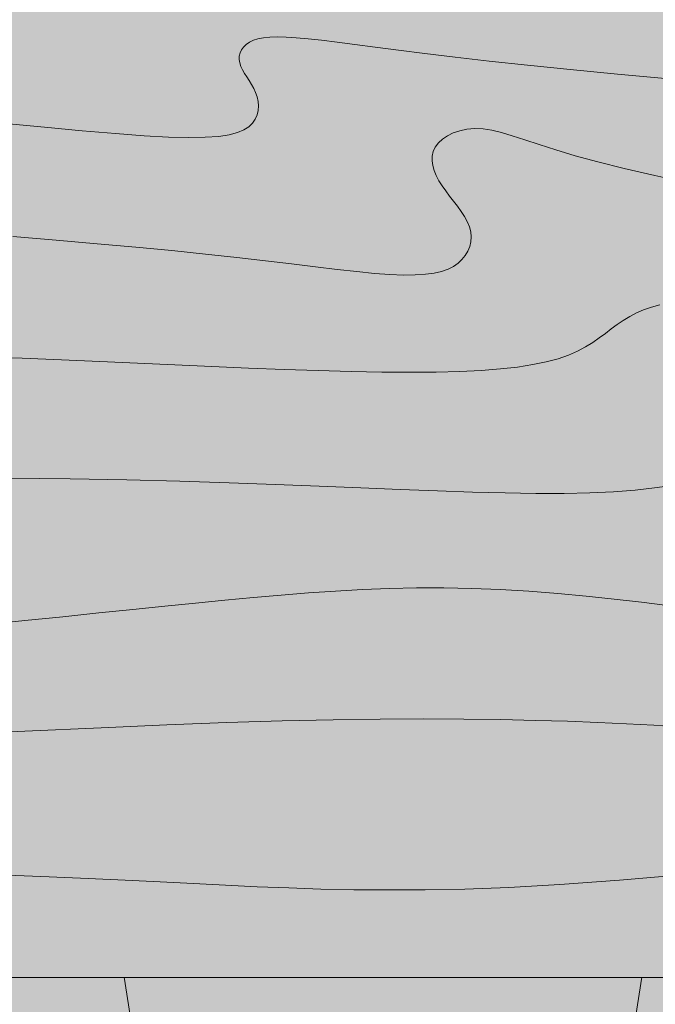
# Model space of a CAD drawing. Units: inches. Extents: x 3024 to 3952, y 1308 to 1863.
# Tile 10 of 29: x 3357 to 3374, y 1587 to 1613. Entities that reach past the tile are written whole.
import ezdxf

# ---------------------------------------------------------------- set-up
doc = ezdxf.new("R2010")
doc.units = ezdxf.units.IN
doc.layers.add('A-FLOR-PATT', color=254, linetype='Continuous', lineweight=13, true_color=0xfeeab9)
for name, color, linetype, lineweight in [('A-FLOR-TILE-PATT', 7, 'Continuous', 13), ('A-FURN', 8, 'Continuous', 18), ('A-FURN-PATT', 9, 'Continuous', 13)]:
    doc.layers.add(name, color=color, linetype=linetype, lineweight=lineweight)

# ---------------------------------------------------------------- blocks, each defined once
blk = doc.blocks.new('Dining Set - 36 x 72 in.')
for p, q in [((-36, -18), (36, -18)), ((5.7657, -26.0006), (4.5153, -17.99762)), ((23.4848, -17.99762), (22.2345, -25.99928))]:
    blk.add_line(p, q)
for points in [[(0.0365, 13.29166), (1.5945, 13.14388), (2.9811, 13.01562), (4.1988, 12.9108), (5.25, 12.83333), (6.1393, 12.78613), (6.8802, 12.76823), (7.4883, 12.77767), (7.9792, 12.8125), (8.3685, 12.87077), (8.6719, 12.95052), (8.9049, 13.0498), (9.0833, 13.16666), (9.2205, 13.29899), (9.3216, 13.44401), (9.3895, 13.59879), (9.4271, 13.76041), (9.4373, 13.92594), (9.4232, 14.09245), (9.3875, 14.257), (9.3333, 14.41666), (9.2638, 14.56917), (9.1836, 14.71484), (9.0975, 14.85465), (9.0104, 14.98958), (8.9272, 15.1206), (8.8529, 15.2487), (8.7922, 15.37483), (8.75, 15.5), (8.7305, 15.62467), (8.7344, 15.74739), (8.7617, 15.86621), (8.8125, 15.97916), (8.8867, 16.08431), (8.9844, 16.17968), (9.1055, 16.26334), (9.25, 16.33333), (9.4189, 16.38802), (9.6172, 16.42708), (9.8506, 16.45052), (10.125, 16.45833), (10.4463, 16.45052), (10.8203, 16.42708), (11.2529, 16.38802), (11.75, 16.33333), (12.3184, 16.26318), (12.9694, 16.17838), (13.7151, 16.07991), (14.5677, 15.96875), (15.5395, 15.84586), (16.6426, 15.71224), (17.8893, 15.56884), (19.2917, 15.41666), (20.859, 15.25667), (22.5879, 15.08984), (24.4721, 14.91715)], [(0.4415, 9.14534), (2.026, 9.01041), (3.5266, 8.87939), (4.9408, 8.7513), (6.266, 8.62516), (7.5, 8.5), (8.6411, 8.37549), (9.6914, 8.2539), (10.6538, 8.13818), (11.5312, 8.03125), (12.3267, 7.93603), (13.043, 7.85547), (13.6831, 7.79248), (14.25, 7.75), (14.7471, 7.7303), (15.1797, 7.73307), (15.5537, 7.75732), (15.875, 7.80208), (16.1494, 7.86637), (16.3828, 7.94922), (16.5811, 8.04964), (16.75, 8.16666), (16.8944, 8.29915), (17.0143, 8.44531), (17.1089, 8.60319), (17.1771, 8.77083), (17.218, 8.94629), (17.2305, 9.1276), (17.2137, 9.31282), (17.1667, 9.5), (17.0895, 9.6875), (16.987, 9.875), (16.8649, 10.0625), (16.7292, 10.25), (16.5856, 10.4375), (16.4401, 10.625), (16.2985, 10.8125), (16.1667, 11), (16.05, 11.18733), (15.9518, 11.3737), (15.8752, 11.5581), (15.8229, 11.73958), (15.798, 11.91715), (15.8034, 12.08984), (15.842, 12.25667), (15.9167, 12.41666), (16.0295, 12.56836), (16.1784, 12.70833), (16.3605, 12.83268), (16.5729, 12.9375), (16.8127, 13.01888), (17.0768, 13.07291), (17.3625, 13.0957), (17.6667, 13.08333), (17.9894, 13.03312), (18.3418, 12.94726), (18.7382, 12.82918), (19.1927, 12.68229), (19.7195, 12.51001), (20.3327, 12.31575), (21.0465, 12.10294), (21.875, 11.875), (22.8357, 11.63354), (23.959, 11.37304), (25.2786, 11.08618)], [(-0.7396, 4.73958), (0.7739, 4.6831), (2.22, 4.6237), (3.6213, 4.56233), (5, 4.5), (6.373, 4.43782), (7.7344, 4.3776), (9.0723, 4.32129), (10.375, 4.27083), (11.6309, 4.22819), (12.8281, 4.19531), (13.9551, 4.17415), (15, 4.16666), (15.954, 4.17448), (16.819, 4.19791), (17.6001, 4.23698), (18.3021, 4.29166), (18.9299, 4.36198), (19.4883, 4.44791), (19.9823, 4.54948), (20.4167, 4.66666), (20.7969, 4.79899), (21.1302, 4.94401), (21.4245, 5.09879), (21.6875, 5.26041), (21.9271, 5.42594), (22.1511, 5.59245), (22.3672, 5.757), (22.5834, 5.91666), (22.8065, 6.06868), (23.0404, 6.21093), (23.2879, 6.34147), (23.5521, 6.45833), (23.8358, 6.55957), (24.142, 6.64323)], [(0.2878, 0.28711), (2.5317, 0.26163), (4.6146, 0.22396), (6.5529, 0.17651), (8.3633, 0.12174), (10.0623, 0.06209), (11.6667, 0), (13.1899, -0.06201), (14.6341, -0.1211), (15.9982, -0.17432), (17.2813, -0.21875), (18.4823, -0.25147), (19.6003, -0.26953), (20.6343, -0.27002), (21.5834, -0.25), (22.4481, -0.20768), (23.2357, -0.14584), (23.9549, -0.06836), (24.6146, 0.02083)], [(-0.625, -5.08334), (0.8708, -4.93099), (2.2715, -4.78646), (3.5872, -4.64974), (4.8281, -4.52084), (6.0046, -4.39974), (7.127, -4.28646), (8.2053, -4.18099), (9.25, -4.08334), (10.2705, -3.99382), (11.2734, -3.91407), (12.2647, -3.84603), (13.25, -3.79167), (14.2354, -3.75293), (15.2266, -3.73177), (16.2295, -3.73015), (17.25, -3.75), (18.2912, -3.79248), (19.3451, -3.85547), (20.4009, -3.93604), (21.4479, -4.03125), (22.4754, -4.13819), (23.4727, -4.25391), (24.4289, -4.37549)], [(-2.5226, -9.12354), (0.8789, -8.98047), (3.6769, -8.85498), (6.0833, -8.75), (8.2767, -8.66765), (10.3021, -8.60677), (12.1712, -8.56543), (13.8958, -8.54167), (15.4876, -8.53353), (16.9583, -8.53907), (18.3197, -8.55632), (19.5834, -8.58334), (20.7616, -8.61841), (21.8685, -8.66081), (22.9188, -8.71004), (23.9271, -8.76563), (24.9081, -8.82707)], [(0.2448, -14.26042), (1.7647, -14.3169), (3.1973, -14.3763), (4.5507, -14.43767), (5.8333, -14.5), (7.0554, -14.5621), (8.235, -14.62175), (9.3922, -14.67652), (10.5469, -14.72396), (11.7192, -14.76164), (12.929, -14.78711), (14.1965, -14.79794), (15.5417, -14.79167), (16.9933, -14.76424), (18.6152, -14.70508), (20.4804, -14.60197), (22.6615, -14.44271), (25.2312, -14.21509), (28.2624, -13.9069), (31.8277, -13.50594), (36, -13)]]:
    blk.add_lwpolyline(points)

msp = doc.modelspace()

# ---------------------------------------------------------------- hatches: boundary and pattern name
at = {"layer": 'A-FLOR-PATT', "transparency": 33554528}
h = msp.add_hatch(color=256, dxfattribs=at)
h.dxf.hatch_style = 1
h.paths.add_polyline_path([(3460.764, 1688.6064), (3412.764, 1688.6064), (3412.764, 1694.6064), (3460.764, 1694.6064), (3460.764, 1778.6064), (3406.764, 1778.6064), (3406.764, 1759.9514), (3318.2981, 1759.9514), (3318.2981, 1658.6064), (3322.5356, 1658.6064), (3322.5356, 1652.6064), (3292.764, 1652.6064), (3292.764, 1778.6064), (3106.764, 1778.6064), (3106.764, 1628.6064), (3172.764, 1628.6064), (3172.764, 1532.6064), (3166.764, 1532.6064), (3166.764, 1628.6064), (3106.764, 1628.6064), (3106.764, 1356.8452), (3202.812, 1356.8452), (3202.812, 1354.2534), (3202.812, 1353.8388), (3202.812, 1351.1212), (3202.812, 1347.8452), (3277.764, 1347.8452), (3277.764, 1353.8452), (3277.764, 1356.8452), (3277.764, 1442.6064), (3460.764, 1442.6064)])
h.paths.add_polyline_path([(3216.238, 1527.2064), (3216.238, 1491.2064), (3214.663, 1491.2064), (3214.663, 1491.2409, -0.3966224), (3180.243, 1526.6064), (3163.0285, 1526.6064), (3163.0285, 1531.1064), (3161.716, 1531.1064), (3161.716, 1561.1064), (3163.0285, 1561.1064), (3163.0285, 1531.1064), (3163.0285, 1526.6064), (3180.243, 1526.6064, 0.3966224), (3214.663, 1491.2409), (3214.663, 1527.2064)], flags=16)
h.paths.add_polyline_path([(3227.364, 1649.8972), (3191.364, 1649.8972), (3191.364, 1651.4722), (3227.364, 1651.4722)], flags=16)
h.paths.add_polyline_path([(3323.1172, 1606.7362), (3323.8545, 1606.8514), (3323.8545, 1594.8241), (3323.1172, 1594.9393)], flags=16)
h.paths.add_polyline_path([(3324.2232, 1606.909), (3330.1216, 1607.8307), (3330.1216, 1614.1093), (3339.3495, 1614.1093), (3340.2711, 1620.0078), (3352.4136, 1620.0078), (3353.3353, 1614.1093), (3359.9941, 1614.1093), (3360.9157, 1620.0078), (3373.0582, 1620.0078), (3373.9799, 1614.1093), (3383.2077, 1614.1093), (3383.2077, 1607.8307), (3389.1062, 1606.909), (3389.1062, 1594.7665), (3383.2077, 1593.8449), (3383.2077, 1587.5663), (3373.9799, 1587.5663), (3373.0583, 1581.6678), (3360.9157, 1581.6678), (3359.9941, 1587.5663), (3353.3353, 1587.5663), (3352.4136, 1581.6678), (3340.2711, 1581.6678), (3339.3495, 1587.5663), (3330.1216, 1587.5663), (3330.1216, 1593.8449), (3324.2232, 1594.7665)], flags=16)
h.paths.add_polyline_path([(3236.1584, 1693.1064), (3236.1584, 1723.1064), (3237.4709, 1723.1064), (3237.4709, 1693.1064)], flags=16)
h.paths.add_polyline_path([(3373.2158, 1600.6847), (3373.7965, 1600.7303), (3374.3268, 1600.7874), (3374.8132, 1600.8531), (3375.2621, 1600.9247), (3375.6801, 1600.9991), (3376.0736, 1601.0735), (3376.6855, 1601.19), (3377.366, 1601.3023), (3378.0667, 1601.3814), (3378.8026, 1601.4123), (3379.5865, 1601.3839), (3380.4537, 1601.2948), (3381.301, 1601.1717), (3382.0317, 1601.0433), (3382.4398, 1600.9607), (3382.6252, 1600.9201), (3382.919, 1600.8507), (3382.9044, 1600.8531), (3382.842, 1600.8678), (3382.7541, 1600.8896), (3382.6252, 1600.9201), (3382.4398, 1600.9607), (3382.1868, 1601.0119), (3381.8738, 1601.0711), (3381.5125, 1601.1346), (3381.1149, 1601.1988), (3380.6928, 1601.2601), (3380.2581, 1601.3149), (3379.8226, 1601.3597), (3379.3984, 1601.3908), (3378.9944, 1601.4054), (3378.6092, 1601.4042), (3378.2384, 1601.3886), (3377.8777, 1601.36), (3377.5227, 1601.32), (3377.1691, 1601.2698), (3376.8127, 1601.211), (3376.4491, 1601.145), (3376.0736, 1601.0735), (3375.4177, 1600.9494), (3374.5542, 1600.8119), (3373.5044, 1600.6988)], flags=0)
h.paths.add_polyline_path([(3380.0253, 1596.7351), (3380.499, 1596.6659), (3380.9706, 1596.6119), (3381.4375, 1596.5791), (3381.8971, 1596.5736), (3382.5886, 1596.6167), (3382.7848, 1596.6692), (3382.1465, 1596.5706), (3381.236, 1596.5815), (3380.3199, 1596.6865)], flags=0)
h.paths.add_polyline_path([(3369.6414, 1603.9617), (3370.1589, 1604.0021), (3370.6218, 1604.0539), (3371.0335, 1604.1173), (3371.3978, 1604.1921), (3371.7181, 1604.2785), (3371.9984, 1604.3761), (3372.2441, 1604.483), (3372.4611, 1604.5972), (3372.655, 1604.7163), (3372.8317, 1604.8384), (3372.9968, 1604.9611), (3373.3703, 1605.2455), (3373.8426, 1605.5328), (3374.4624, 1605.7539), (3375.1058, 1605.8302), (3375.7221, 1605.8261), (3376.4109, 1605.76), (3377.1534, 1605.6376), (3377.8945, 1605.473), (3378.1382, 1605.409), (3377.7394, 1605.5074), (3377.3509, 1605.5937), (3376.9704, 1605.6677), (3376.5999, 1605.7288), (3376.2417, 1605.7762), (3375.8979, 1605.8092), (3375.5707, 1605.8271), (3375.2621, 1605.8291), (3374.9745, 1605.8146), (3374.7092, 1605.7832), (3374.4647, 1605.7359), (3374.239, 1605.6742), (3374.0298, 1605.5996), (3373.835, 1605.5134), (3373.6525, 1605.4171), (3373.4801, 1605.3123), (3373.3156, 1605.2002), (3373.1562, 1605.0825), (3372.7603, 1604.781), (3372.236, 1604.4588), (3371.5738, 1604.2283), (3370.8493, 1604.0794), (3369.9262, 1603.976)], flags=0)
h.paths.add_polyline_path([(3366.7533, 1606.5832), (3367.1713, 1606.5519), (3367.5378, 1606.5374), (3367.8568, 1606.5394), (3368.1325, 1606.5573), (3368.3694, 1606.5903), (3368.5717, 1606.6377), (3368.7438, 1606.6988), (3368.89, 1606.7728), (3369.0146, 1606.8591), (3369.121, 1606.9568), (3369.2094, 1607.0646), (3369.2792, 1607.181), (3369.3295, 1607.3046), (3369.3596, 1607.4339), (3369.3688, 1607.5676), (3369.3565, 1607.7042), (3369.3218, 1607.8422), (3369.2649, 1607.9804), (3369.1893, 1608.1187), (3369.0993, 1608.2569), (3368.9992, 1608.3952), (3368.8934, 1608.5334), (3368.7861, 1608.6717), (3368.6817, 1608.8099), (3368.4212, 1609.1804), (3368.2685, 1609.7106), (3368.4883, 1610.1814), (3369.0537, 1610.4604), (3369.6717, 1610.5097), (3370.2812, 1610.3612), (3370.4805, 1610.2968), (3370.1882, 1610.3839), (3369.9284, 1610.4472), (3369.6905, 1610.4842), (3369.4662, 1610.4933), (3369.2555, 1610.4765), (3369.0608, 1610.4367), (3368.884, 1610.3767), (3368.7274, 1610.2994), (3368.5931, 1610.2077), (3368.4833, 1610.1045), (3368.4002, 1609.9927), (3368.3451, 1609.8747), (3368.3166, 1609.7517), (3368.3127, 1609.6244), (3368.331, 1609.4935), (3368.3696, 1609.3597), (3368.4261, 1609.2237), (3368.4985, 1609.0863), (3368.5845, 1608.9482), (3368.6817, 1608.8099), (3368.7861, 1608.6717), (3368.8934, 1608.5334), (3368.9992, 1608.3952), (3369.0993, 1608.2569), (3369.3398, 1607.8876), (3369.3941, 1607.2896), (3368.9774, 1606.7817), (3368.3928, 1606.5742), (3367.7162, 1606.5303), (3367.0044, 1606.5585)], flags=0)
h.paths.add_polyline_path([(3362.1859, 1610.2589), (3362.5478, 1610.2845), (3362.8348, 1610.3275), (3363.0585, 1610.3863), (3363.2303, 1610.4595), (3363.3619, 1610.5457), (3363.463, 1610.6432), (3363.5376, 1610.7502), (3363.5876, 1610.8643), (3363.6153, 1610.9834), (3363.6229, 1611.1055), (3363.6125, 1611.2283), (3363.5861, 1611.3496), (3363.5462, 1611.4673), (3363.4949, 1611.5797), (3363.4358, 1611.6871), (3363.3723, 1611.7902), (3363.3081, 1611.8897), (3363.2468, 1611.9863), (3363.192, 1612.0808), (3363.0258, 1612.4261), (3363.3371, 1612.8672), (3363.9008, 1612.9782), (3364.4822, 1612.9641), (3365.1098, 1612.9074), (3365.328, 1612.8805), (3364.9615, 1612.9208), (3364.6426, 1612.9496), (3364.3668, 1612.9669), (3364.1299, 1612.9726), (3363.9276, 1612.9669), (3363.7555, 1612.9496), (3363.6093, 1612.9208), (3363.4848, 1612.8805), (3363.3782, 1612.8289), (3363.2889, 1612.7672), (3363.2169, 1612.6969), (3363.1622, 1612.6193), (3363.1247, 1612.5361), (3363.1046, 1612.4484), (3363.1017, 1612.358), (3363.1161, 1612.266), (3363.1472, 1612.1738), (3363.192, 1612.0808), (3363.2468, 1611.9863), (3363.3081, 1611.8897), (3363.3723, 1611.7902), (3363.4358, 1611.6871), (3363.6363, 1611.323), (3363.5979, 1610.7003), (3363.0863, 1610.3651), (3362.3983, 1610.2622)], flags=0)
h.paths.add_polyline_path([(3352.356, 1581.2991), (3352.2408, 1580.5618), (3340.4439, 1580.5618), (3340.3287, 1581.2991)], flags=16)
h.paths.add_polyline_path([(3340.4439, 1621.1137), (3352.2408, 1621.1137), (3352.356, 1620.3764), (3340.3287, 1620.3764)], flags=16)
h.paths.add_polyline_path([(3278.4282, 1504.7424), (3290.3831, 1504.7424), (3290.3831, 1502.7499), (3291.0473, 1502.7499), (3291.0473, 1494.7799), (3290.3831, 1494.7799), (3290.3831, 1494.1158), (3291.0473, 1494.1158), (3291.0473, 1486.1458), (3290.3831, 1486.1458), (3290.3831, 1484.1533), (3291.0473, 1484.1533), (3291.0473, 1483.4892, -0.0909091), (3291.0473, 1468.8776), (3291.0473, 1468.2135), (3290.3831, 1468.2135), (3290.3831, 1464.8926), (3278.4282, 1464.8926), (3278.4282, 1472.8626), (3277.764, 1473.5268), (3277.764, 1478.84), (3278.4282, 1479.5042)], flags=16)
h.paths.add_polyline_path([(3278.7603, 1504.4103), (3290.051, 1504.4103), (3290.051, 1465.2247), (3278.7603, 1465.2247)], flags=0)
h.paths.add_polyline_path([(3123.904, 1600.7821), (3117.9039, 1602.7821), (3117.9039, 1599.7821), (3119.4039, 1599.7821), (3119.4039, 1596.7821), (3118.4039, 1596.7821), (3118.4039, 1598.7821), (3117.9039, 1598.7821), (3117.9039, 1596.2821), (3109.9039, 1596.2821), (3109.9039, 1617.2821), (3117.9039, 1617.2821), (3117.9039, 1610.7821), (3123.9038, 1612.7821, -0.7025712), (3137.9039, 1606.7822, -0.7025621)], flags=16)
h.paths.add_polyline_path([(3123.9039, 1602.7822), (3123.9039, 1610.7822, -0.7345333), (3136.9039, 1606.7822, -0.7345297)], flags=0)
h.paths.add_polyline_path([(3177.972, 1689.6473), (3109.2405, 1689.6473), (3109.2405, 1741.1959), (3177.972, 1741.1959)], flags=16)
h.paths.add_polyline_path([(3373.0006, 1581.2991), (3372.8854, 1580.5618), (3361.0885, 1580.5618), (3360.9733, 1581.2991)], flags=16)
h.paths.add_polyline_path([(3361.0885, 1621.1137), (3372.8854, 1621.1137), (3373.0006, 1620.3764), (3360.9733, 1620.3764)], flags=16)
h.paths.add_polyline_path([(3116.9039, 1598.2821, -0.4142136), (3116.1539, 1597.2821), (3111.9039, 1597.2821, -0.4142136), (3110.9039, 1598.0321), (3110.9039, 1615.2821, -0.4142136), (3111.6539, 1616.2821), (3115.9039, 1616.2821, -0.4142136), (3116.9039, 1615.5321)], flags=0)
h.paths.add_polyline_path([(3121.6122, 1728.1369), (3121.6122, 1696.5205), (3110.2715, 1696.5205), (3110.2715, 1714.3906), (3121.6122, 1714.3906), (3121.6122, 1716.4526), (3110.2715, 1716.4526), (3110.2715, 1734.3228), (3123.3304, 1734.3228), (3123.3304, 1729.8552), (3134.6711, 1741.1959), (3134.6711, 1728.1369)], flags=0)
h.paths.add_polyline_path([(3389.4748, 1606.8514), (3390.2122, 1606.7362), (3390.2122, 1594.9393), (3389.4748, 1594.8241)], flags=16)
h.paths.add_polyline_path([(3257.6842, 1762.8281), (3259.6842, 1768.8281), (3256.6842, 1768.8281), (3256.6842, 1767.3281), (3253.6842, 1767.3281), (3253.6842, 1768.3281), (3255.6842, 1768.3281), (3255.6842, 1768.8281), (3253.1842, 1768.8281), (3253.1842, 1776.8281), (3274.1842, 1776.8281), (3274.1842, 1768.8281), (3267.6842, 1768.8281), (3269.6842, 1762.8282, -0.7025712), (3263.6843, 1748.8282, -0.7025621)], flags=16)
h.paths.add_polyline_path([(3259.6842, 1762.8281), (3267.6843, 1762.8281, -0.7345333), (3263.6842, 1749.8282, -0.7345297)], flags=0)
h.paths.add_polyline_path([(3411.264, 1715.6064), (3411.264, 1716.9189), (3441.264, 1716.9189), (3441.264, 1715.6064)], flags=16)
h.paths.add_polyline_path([(3178.3806, 1449.1876), (3178.3806, 1397.639), (3109.6491, 1397.639), (3109.6491, 1449.1876)], flags=16)
h.paths.add_polyline_path([(3397.1501, 1541.7146), (3419.6183, 1541.7146), (3419.6183, 1496.7783), (3397.1501, 1496.7783)], flags=16)
h.paths.add_polyline_path([(3254.1842, 1770.5781), (3254.1842, 1774.8281, -0.4142136), (3254.9342, 1775.8281), (3272.1842, 1775.8281, -0.4142136), (3273.1842, 1775.0781), (3273.1842, 1770.8281, -0.4142136), (3272.4342, 1769.8281), (3255.1842, 1769.8281, -0.4142136)], flags=0)
h.paths.add_polyline_path([(3403.672, 1500.7601), (3403.6016, 1500.3997), (3403.5328, 1500.0441), (3403.4662, 1499.6867), (3403.4027, 1499.3226), (3403.3464, 1498.9532), (3403.3025, 1498.5811), (3403.2759, 1498.2091), (3403.2714, 1497.8401), (3403.3064, 1497.2813), (3403.3491, 1497.1219), (3403.2689, 1497.6395), (3403.2778, 1498.3719), (3403.3635, 1499.0984), (3403.4889, 1499.8168), (3403.6016, 1500.3997), (3403.672, 1500.7601), (3403.744, 1501.1315), (3403.817, 1501.5205), (3403.891, 1501.9336), (3403.9656, 1502.3769), (3404.0404, 1502.8572), (3404.115, 1503.3786), (3404.2264, 1504.2311), (3404.2571, 1504.5223), (3404.1552, 1503.6598), (3404.0063, 1502.6193), (3403.8604, 1501.7518), (3403.744, 1501.1315)], flags=0)
h.paths.add_polyline_path([(3406.5868, 1505.0416), (3406.6121, 1504.5236), (3406.6492, 1504.0526), (3406.6956, 1503.624), (3406.7491, 1503.2333), (3406.8072, 1502.8759), (3406.8676, 1502.5473), (3406.9281, 1502.243), (3407.0268, 1501.7597), (3407.1416, 1501.1368), (3407.2087, 1500.3904), (3407.1804, 1499.6703), (3407.1078, 1498.9956), (3407.0074, 1498.3199), (3406.8809, 1497.6059), (3406.7403, 1496.9627), (3406.7418, 1496.9824), (3406.7491, 1497.0249), (3406.8229, 1497.3409), (3406.8364, 1497.4025), (3406.878, 1497.6078), (3406.9261, 1497.8614), (3406.9777, 1498.1526), (3407.0298, 1498.4712), (3407.0797, 1498.8068), (3407.1243, 1499.149), (3407.1607, 1499.4874), (3407.1859, 1499.8115), (3407.1978, 1500.1137), (3407.1969, 1500.3962), (3407.1841, 1500.6642), (3407.1609, 1500.9225), (3407.1284, 1501.1761), (3407.0876, 1501.43), (3407.0398, 1501.6891), (3406.9862, 1501.9585), (3406.8832, 1502.4628), (3406.7712, 1503.0713), (3406.6657, 1503.8424), (3406.5924, 1504.7735)], flags=0)
h.paths.add_polyline_path([(3409.2517, 1507.8962), (3409.2752, 1507.4282), (3409.3079, 1507.0076), (3409.3501, 1506.6314), (3409.4015, 1506.2969), (3409.4624, 1506.0009), (3409.5326, 1505.7406), (3409.6119, 1505.5128), (3409.6988, 1505.3131), (3409.7915, 1505.1368), (3409.8883, 1504.9792), (3409.9875, 1504.8356), (3410.0872, 1504.7015), (3410.1859, 1504.572), (3410.4508, 1504.2132), (3410.7205, 1503.6035), (3410.8059, 1502.8824), (3410.7619, 1502.0875), (3410.6122, 1501.2299), (3410.4402, 1500.6169), (3410.2538, 1500.0031), (3410.0536, 1499.3219), (3409.9909, 1499.0812), (3410.1761, 1499.7472), (3410.3596, 1500.3513), (3410.4512, 1500.6561), (3410.5312, 1500.9412), (3410.6013, 1501.226), (3410.6614, 1501.512), (3410.7111, 1501.7964), (3410.7496, 1502.0763), (3410.7764, 1502.3489), (3410.7909, 1502.6114), (3410.7926, 1502.8608), (3410.7808, 1503.0944), (3410.7553, 1503.31), (3410.7169, 1503.5087), (3410.6667, 1503.6921), (3410.6061, 1503.8621), (3410.5361, 1504.0203), (3410.4578, 1504.1686), (3410.3726, 1504.3088), (3410.2815, 1504.4424), (3410.1859, 1504.572), (3410.0872, 1504.7015), (3409.859, 1505.0083), (3409.5943, 1505.5117), (3409.4266, 1506.1336), (3409.324, 1506.8011), (3409.2586, 1507.6407)], flags=0)
h.paths.add_polyline_path([(3411.4914, 1510.5878), (3411.4432, 1510.1586), (3411.4054, 1509.775), (3411.38, 1509.4354), (3411.3681, 1509.1376), (3411.3698, 1508.8784), (3411.3843, 1508.6542), (3411.4112, 1508.4618), (3411.4497, 1508.2974), (3411.4994, 1508.1575), (3411.5595, 1508.0388), (3411.6296, 1507.9375), (3411.7097, 1507.851), (3411.802, 1507.7792), (3411.9096, 1507.7225), (3412.0353, 1507.6817), (3412.1821, 1507.6572), (3412.3528, 1507.6496), (3412.5505, 1507.6597), (3412.778, 1507.6879), (3413.0364, 1507.7341), (3413.3194, 1507.7955), (3413.6188, 1507.8687), (3413.9264, 1507.95), (3414.234, 1508.036), (3414.5333, 1508.1232), (3414.8163, 1508.208), (3415.0747, 1508.287), (3415.3023, 1508.3569), (3415.5007, 1508.4158), (3415.6733, 1508.4617), (3416.1158, 1508.5538), (3416.512, 1508.2591), (3416.716, 1507.6581), (3416.61, 1507.0003), (3416.3052, 1506.3411), (3415.8928, 1505.618), (3415.7339, 1505.3633), (3415.9914, 1505.791), (3416.201, 1506.1583), (3416.3666, 1506.4739), (3416.4925, 1506.7462), (3416.5828, 1506.9838), (3416.6413, 1507.1949), (3416.6725, 1507.3883), (3416.6799, 1507.5705), (3416.6662, 1507.7417), (3416.6339, 1507.9), (3416.5851, 1508.0436), (3416.5223, 1508.1709), (3416.4478, 1508.28), (3416.3639, 1508.3692), (3416.273, 1508.4368), (3416.1765, 1508.4815), (3416.0718, 1508.5047), (3415.9553, 1508.5079), (3415.8237, 1508.493), (3415.6733, 1508.4617), (3415.5007, 1508.4158), (3415.3327, 1508.3659), (3414.6495, 1508.157), (3414.0606, 1507.9855), (3413.4456, 1507.8229), (3412.8838, 1507.701), (3412.5505, 1507.6597), (3412.0748, 1507.6354), (3411.595, 1507.8883), (3411.398, 1508.4429), (3411.3624, 1508.9927), (3411.3854, 1509.5711), (3411.4578, 1510.3071)], flags=0)
h.paths.add_polyline_path([(3135.0797, 1449.1876), (3135.0797, 1436.1286), (3122.0208, 1436.1286), (3122.0208, 1404.5122), (3110.6801, 1404.5122), (3110.6801, 1422.3823), (3122.0208, 1422.3823), (3122.0208, 1424.4443), (3110.6801, 1424.4443), (3110.6801, 1442.3145), (3123.739, 1442.3145), (3123.739, 1437.8469)], flags=0)
h.paths.add_polyline_path([(3416.4944, 1514.2949), (3416.4837, 1513.8511), (3416.4893, 1513.4867), (3416.5102, 1513.1926), (3416.5451, 1512.9593), (3416.5929, 1512.7775), (3416.6524, 1512.6379), (3416.7224, 1512.531), (3416.8017, 1512.4488), (3416.8886, 1512.3882), (3416.9813, 1512.3476), (3417.0781, 1512.3251), (3417.1773, 1512.3189), (3417.277, 1512.3274), (3417.3757, 1512.3488), (3417.4713, 1512.3813), (3417.5627, 1512.4229), (3417.65, 1512.471), (3417.7338, 1512.5225), (3417.8146, 1512.5747), (3417.8931, 1512.6245), (3417.9699, 1512.6691), (3418.2968, 1512.8265), (3418.6505, 1512.4645), (3418.7037, 1511.9342), (3418.6693, 1511.3839), (3418.6076, 1510.8228), (3418.5777, 1510.5927), (3418.6197, 1510.9333), (3418.6525, 1511.2311), (3418.6759, 1511.4903), (3418.6899, 1511.7144), (3418.6946, 1511.9069), (3418.6899, 1512.0713), (3418.6759, 1512.2112), (3418.6525, 1512.33), (3418.6197, 1512.4311), (3418.5778, 1512.5177), (3418.5276, 1512.5903), (3418.4705, 1512.6488), (3418.4075, 1512.6933), (3418.3399, 1512.7237), (3418.2686, 1512.7401), (3418.1951, 1512.7424), (3418.1204, 1512.7307), (3418.0455, 1512.7055), (3417.9792, 1512.6736), (3417.65, 1512.471), (3417.5627, 1512.4229), (3417.4713, 1512.3813), (3417.3757, 1512.3488), (3417.277, 1512.3274), (3416.878, 1512.2936), (3416.5757, 1512.7549), (3416.492, 1513.3145), (3416.4808, 1514.0384)], flags=0)
h.paths.add_polyline_path([(3392.8223, 1481.9454), (3396.7707, 1481.9454), (3396.7707, 1480.9201), (3428.3585, 1480.9201), (3428.3585, 1481.9454), (3432.3069, 1481.9454), (3432.3069, 1464.8354, -0.266667), (3392.8223, 1464.8354)], flags=16)
h.paths.add_polyline_path([(3431.203, 1547.5428), (3450.8613, 1547.5428, -0.1904762), (3450.8614, 1484.031), (3431.203, 1484.031), (3431.203, 1488.5675), (3432.3809, 1488.5675), (3432.3809, 1543.0062), (3431.203, 1543.0062)], flags=16)
h.paths.add_polyline_path([(3451.9233, 1524.86, -0.0496282), (3451.9233, 1506.7138), (3446.7921, 1506.7138), (3446.7921, 1524.86)], flags=0)
h.paths.add_polyline_path([(3460.764, 1436.6064), (3277.764, 1436.6064), (3277.764, 1356.8452), (3277.764, 1353.8452), (3460.764, 1353.8452)], flags=17)
h.paths.add_polyline_path([(3121.3033, 1577.378), (3153.693, 1577.378), (3153.693, 1586.6752), (3121.3033, 1586.6752)], flags=24)
h.paths.add_polyline_path([(3164.1457, 1464.1276), (3210.4801, 1464.1276), (3210.4801, 1473.4247), (3164.1457, 1473.4247)], flags=24)
h.paths.add_polyline_path([(3343.1909, 1505.8863), (3373.7236, 1505.8863), (3373.7236, 1515.1773), (3343.1909, 1515.1773)], flags=24)
h.paths.add_polyline_path([(3337.6353, 1564.2926), (3370.0189, 1564.2926), (3370.0189, 1573.5836), (3337.6353, 1573.5836)], flags=24)
h.paths.add_polyline_path([(3419.204, 1753.8578), (3453.3997, 1753.8578), (3453.3997, 1762.9956), (3419.204, 1762.9956)], flags=24)
h.paths.add_polyline_path([(3341.2523, 1701.0246), (3381.0761, 1701.0246), (3381.0761, 1710.3156), (3341.2523, 1710.3156)], flags=24)
h.paths.add_polyline_path([(3245.8895, 1726.2997), (3278.2793, 1726.2997), (3278.2793, 1735.5968), (3245.8895, 1735.5968)], flags=24)
h.paths.add_polyline_path([(3128.8045, 1668.6736), (3175.1389, 1668.6736), (3175.1389, 1677.9707), (3128.8045, 1677.9707)], flags=24)
h.paths.add_polyline_path([(3345.9997, 1396.0062), (3389.09, 1396.0062), (3389.09, 1405.3033), (3345.9997, 1405.3033)], flags=24)
at = {"layer": 'A-FLOR-TILE-PATT', "transparency": 33554569}
h = msp.add_hatch(dxfattribs=at)
h.set_pattern_fill('ANGLE', color=256, scale=2)
h.set_pattern_definition([(0, (0, 0), (0, 13.97), [10.16, -3.81]), (90, (0, 0), (-13.97, 9e-16), [10.16, -3.81])])
h.paths.add_polyline_path([(3292.764, 1778.6064), (3232.764, 1778.6064), (3232.764, 1694.6064), (3236.1584, 1694.6064), (3236.1584, 1723.1064), (3237.4709, 1723.1064), (3237.4709, 1723.0777, -0.3870039), (3266.1209, 1694.6064), (3292.764, 1694.6064)])
h.paths.add_polyline_path([(3263.6843, 1748.8282, -0.7025621), (3257.6842, 1762.8281), (3259.6842, 1768.8281), (3256.6842, 1768.8281), (3256.6842, 1767.3281), (3253.6842, 1767.3281), (3253.6842, 1768.3281), (3255.6842, 1768.3281), (3255.6842, 1768.8281), (3253.1842, 1768.8281), (3253.1842, 1776.8281), (3274.1842, 1776.8281), (3274.1842, 1768.8281), (3267.6842, 1768.8281), (3269.6842, 1762.8282, -0.7025712)], flags=16)
h.paths.add_polyline_path([(3263.6842, 1749.8282, -0.7345297), (3259.6842, 1762.8281), (3267.6843, 1762.8281, -0.7345333)], flags=0)
h.paths.add_polyline_path([(3255.1842, 1769.8281, -0.4142136), (3254.1842, 1770.5781), (3254.1842, 1774.8281, -0.4142136), (3254.9342, 1775.8281), (3272.1842, 1775.8281, -0.4142136), (3273.1842, 1775.0781), (3273.1842, 1770.8281, -0.4142136), (3272.4342, 1769.8281)], flags=0)
h.paths.add_polyline_path([(3460.764, 1436.6064), (3277.764, 1436.6064), (3277.764, 1356.8452), (3277.764, 1353.8452), (3460.764, 1353.8452)])
h.paths.add_polyline_path([(3166.764, 1628.6064), (3106.764, 1628.6064), (3106.764, 1532.6064), (3133.066, 1532.6064, -0.3870039), (3161.716, 1561.0777), (3161.716, 1561.1064), (3163.0285, 1561.1064), (3163.0285, 1532.6064), (3166.764, 1532.6064)])
h.paths.add_polyline_path([(3123.904, 1600.7821), (3117.9039, 1602.7821), (3117.9039, 1599.7821), (3119.4039, 1599.7821), (3119.4039, 1596.7821), (3118.4039, 1596.7821), (3118.4039, 1598.7821), (3117.9039, 1598.7821), (3117.9039, 1596.2821), (3109.9039, 1596.2821), (3109.9039, 1617.2821), (3117.9039, 1617.2821), (3117.9039, 1610.7821), (3123.9038, 1612.7821, -0.7025712), (3137.9039, 1606.7822, -0.7025621)], flags=16)
h.paths.add_polyline_path([(3123.9039, 1602.7822), (3123.9039, 1610.7822, -0.7345333), (3136.9039, 1606.7822, -0.7345297)], flags=0)
h.paths.add_polyline_path([(3116.1539, 1597.2821), (3111.9039, 1597.2821, -0.4142136), (3110.9039, 1598.0321), (3110.9039, 1615.2821, -0.4142136), (3111.6539, 1616.2821), (3115.9039, 1616.2821, -0.4142136), (3116.9039, 1615.5321), (3116.9039, 1598.2821, -0.4142136)], flags=0)
h.paths.add_polyline_path([(3245.8895, 1726.2997), (3278.2793, 1726.2997), (3278.2793, 1735.5968), (3245.8895, 1735.5968)], flags=24)
h.paths.add_polyline_path([(3345.9997, 1396.0062), (3389.09, 1396.0062), (3389.09, 1405.3033), (3345.9997, 1405.3033)], flags=24)
h.paths.add_polyline_path([(3121.3033, 1577.378), (3153.693, 1577.378), (3153.693, 1586.6752), (3121.3033, 1586.6752)], flags=24)
at = {"layer": 'A-FURN-PATT', "transparency": 33554511}
h = msp.add_hatch(color=256, dxfattribs=at)
h.dxf.hatch_style = 1
h.paths.add_polyline_path([(3373.0582, 1620.0078), (3360.9157, 1620.0078), (3359.9941, 1614.1093), (3373.9799, 1614.1093)])
h.paths.add_polyline_path([(3372.8854, 1621.1137), (3361.0885, 1621.1137), (3360.9733, 1620.3764), (3373.0006, 1620.3764)])
h.paths.add_polyline_path([(3389.1062, 1606.909), (3383.2077, 1607.8307), (3383.2077, 1593.8449), (3389.1062, 1594.7665)])
h.paths.add_polyline_path([(3390.2122, 1606.7362), (3389.4748, 1606.8514), (3389.4748, 1594.8241), (3390.2122, 1594.9393)])
h.paths.add_polyline_path([(3373.9799, 1587.5663), (3359.9941, 1587.5663), (3360.9157, 1581.6678), (3373.0583, 1581.6678)])
h.paths.add_polyline_path([(3373.0006, 1581.2991), (3360.9733, 1581.2991), (3361.0885, 1580.5618), (3372.8854, 1580.5618)])
h.paths.add_polyline_path([(3353.3353, 1587.5663), (3339.3495, 1587.5663), (3340.2711, 1581.6678), (3352.4136, 1581.6678)])
h.paths.add_polyline_path([(3352.356, 1581.2991), (3340.3287, 1581.2991), (3340.4439, 1580.5618), (3352.2408, 1580.5618)])
h.paths.add_polyline_path([(3330.1216, 1607.8307), (3324.2232, 1606.909), (3324.2232, 1594.7665), (3330.1216, 1593.8449)])
h.paths.add_polyline_path([(3323.8545, 1606.8514), (3323.1172, 1606.7362), (3323.1172, 1594.9393), (3323.8545, 1594.8241)])
h.paths.add_polyline_path([(3352.4136, 1620.0078), (3340.2711, 1620.0078), (3339.3495, 1614.1093), (3353.3353, 1614.1093)])
h.paths.add_polyline_path([(3352.2408, 1621.1137), (3340.4439, 1621.1137), (3340.3287, 1620.3764), (3352.356, 1620.3764)])
at = {"layer": 'A-FURN-PATT', "transparency": 33554600}
h = msp.add_hatch(color=256, dxfattribs=at)
h.dxf.hatch_style = 1
h.paths.add_polyline_path([(3363.5462, 1611.4673), (3363.4949, 1611.5797), (3363.4358, 1611.6871), (3363.3723, 1611.7902), (3363.2557, 1611.9708), (3363.16, 1612.1359), (3363.1003, 1612.3129), (3363.1061, 1612.4946), (3363.1815, 1612.6623), (3363.3264, 1612.8038), (3363.5397, 1612.9071), (3363.7555, 1612.9496), (3363.9276, 1612.9669), (3364.1299, 1612.9726), (3364.3668, 1612.9669), (3364.6426, 1612.9496), (3364.9615, 1612.9208), (3365.328, 1612.8805), (3365.7471, 1612.8287), (3366.2271, 1612.7662), (3366.7769, 1612.6936), (3367.4055, 1612.6117), (3368.1221, 1612.5211), (3368.9354, 1612.4225), (3369.8546, 1612.3168), (3370.8886, 1612.2046), (3372.0442, 1612.0866), (3373.3189, 1611.9636), (3374.7081, 1611.8363), (3376.2072, 1611.7054), (3377.8113, 1611.5716), (3379.516, 1611.4356), (3381.3163, 1611.2982), (3383.2077, 1611.1601), (3383.2077, 1614.1093), (3330.1216, 1614.1093), (3330.1216, 1611.8974), (3333.6775, 1611.8808), (3336.899, 1611.834), (3339.8144, 1611.7613), (3342.4523, 1611.667), (3344.8411, 1611.5554), (3347.0091, 1611.4308), (3348.985, 1611.2976), (3350.797, 1611.1601), (3352.4691, 1611.0223), (3354.0078, 1610.8874), (3355.4146, 1610.7583), (3356.6916, 1610.6378), (3357.8403, 1610.5289), (3358.8627, 1610.4343), (3359.7605, 1610.357), (3360.5355, 1610.2999), (3361.1912, 1610.2651), (3361.7375, 1610.2519), (3362.1859, 1610.2589), (3362.5478, 1610.2845), (3362.8348, 1610.3275), (3363.0585, 1610.3863), (3363.2303, 1610.4595), (3363.3619, 1610.5457), (3363.463, 1610.6432), (3363.5376, 1610.7502), (3363.5876, 1610.8643), (3363.6153, 1610.9834), (3363.6229, 1611.1055), (3363.6125, 1611.2283), (3363.5861, 1611.3496)])
h.paths.add_polyline_path([(3368.8934, 1608.5334), (3368.7093, 1608.7706), (3368.5315, 1609.0235), (3368.3879, 1609.2961), (3368.3108, 1609.5637), (3368.3187, 1609.8182), (3368.4002, 1609.9927), (3368.4833, 1610.1045), (3368.5931, 1610.2077), (3368.7274, 1610.2994), (3368.884, 1610.3767), (3369.0608, 1610.4367), (3369.2555, 1610.4765), (3369.4662, 1610.4933), (3369.6905, 1610.4842), (3369.9284, 1610.4472), (3370.1882, 1610.3839), (3370.4805, 1610.2968), (3370.8156, 1610.1885), (3371.204, 1610.0615), (3371.6561, 1609.9183), (3372.1824, 1609.7614), (3372.7933, 1609.5933), (3373.5016, 1609.4153), (3374.3298, 1609.2232), (3375.3028, 1609.0117), (3376.4453, 1608.7754), (3377.7822, 1608.5088), (3379.3383, 1608.2065), (3381.1386, 1607.8633), (3383.2077, 1607.4735), (3383.2077, 1611.1601), (3381.3163, 1611.2982), (3379.516, 1611.4356), (3377.8113, 1611.5716), (3376.2072, 1611.7054), (3374.7081, 1611.8363), (3373.3189, 1611.9636), (3372.0442, 1612.0866), (3370.8886, 1612.2046), (3369.8546, 1612.3168), (3368.9354, 1612.4225), (3368.1221, 1612.5211), (3367.4055, 1612.6117), (3366.7769, 1612.6936), (3366.2271, 1612.7662), (3365.7471, 1612.8287), (3365.328, 1612.8805), (3364.9615, 1612.9208), (3364.6426, 1612.9496), (3364.3668, 1612.9669), (3364.1299, 1612.9726), (3363.9276, 1612.9669), (3363.7555, 1612.9496), (3363.6093, 1612.9208), (3363.4848, 1612.8805), (3363.3782, 1612.8289), (3363.2889, 1612.7672), (3363.2169, 1612.6969), (3363.1622, 1612.6193), (3363.1247, 1612.5361), (3363.1046, 1612.4484), (3363.1017, 1612.358), (3363.1161, 1612.266), (3363.1472, 1612.1738), (3363.192, 1612.0808), (3363.2468, 1611.9863), (3363.3081, 1611.8897), (3363.4181, 1611.7194), (3363.529, 1611.5178), (3363.6075, 1611.2866), (3363.6284, 1611.0397), (3363.5728, 1610.8008), (3363.4229, 1610.5856), (3363.2303, 1610.4595), (3363.0585, 1610.3863), (3362.8348, 1610.3275), (3362.5478, 1610.2845), (3362.1859, 1610.2589), (3361.7375, 1610.2519), (3361.1912, 1610.2651), (3360.5355, 1610.2999), (3359.7605, 1610.357), (3358.8627, 1610.4343), (3357.8403, 1610.5289), (3356.6916, 1610.6378), (3355.4146, 1610.7583), (3354.0078, 1610.8874), (3352.4691, 1611.0223), (3350.797, 1611.1601), (3348.985, 1611.2976), (3347.0091, 1611.4308), (3344.8411, 1611.5554), (3342.4523, 1611.667), (3339.8144, 1611.7613), (3336.899, 1611.834), (3333.6775, 1611.8808), (3330.1216, 1611.8974), (3330.1216, 1608.2109), (3335.3, 1608.3161), (3339.5794, 1608.3616), (3343.0805, 1608.3567), (3345.9238, 1608.3107), (3348.23, 1608.2331), (3350.1196, 1608.1331), (3351.7134, 1608.0202), (3353.1317, 1607.9036), (3354.475, 1607.7912), (3355.7618, 1607.6838), (3356.9902, 1607.5807), (3358.1585, 1607.4812), (3359.2649, 1607.3846), (3360.3076, 1607.2902), (3361.2846, 1607.1972), (3362.1945, 1607.1049), (3363.0358, 1607.0131), (3363.8102, 1606.9234), (3364.5198, 1606.8381), (3365.1667, 1606.7593), (3365.7532, 1606.6891), (3366.2814, 1606.6297), (3366.7533, 1606.5832), (3367.1713, 1606.5519), (3367.5378, 1606.5374), (3367.8568, 1606.5394), (3368.1325, 1606.5573), (3368.3694, 1606.5903), (3368.5717, 1606.6377), (3368.7438, 1606.6988), (3368.89, 1606.7728), (3369.0146, 1606.8591), (3369.121, 1606.9568), (3369.2094, 1607.0646), (3369.2792, 1607.181), (3369.3295, 1607.3046), (3369.3596, 1607.4339), (3369.3688, 1607.5676), (3369.3565, 1607.7042), (3369.3218, 1607.8422), (3369.2649, 1607.9804), (3369.1893, 1608.1187), (3369.0993, 1608.2569), (3368.9992, 1608.3952)])
h.paths.add_polyline_path([(3374.239, 1605.6742), (3374.4647, 1605.7359), (3374.7092, 1605.7832), (3374.9745, 1605.8146), (3375.2621, 1605.8291), (3375.5707, 1605.8271), (3375.8979, 1605.8092), (3376.2417, 1605.7762), (3376.5999, 1605.7288), (3376.9704, 1605.6677), (3377.3509, 1605.5937), (3377.7394, 1605.5074), (3378.1382, 1605.409), (3378.5679, 1605.2962), (3379.0538, 1605.1661), (3379.621, 1605.0159), (3380.2949, 1604.8426), (3381.1005, 1604.6434), (3382.0631, 1604.4154), (3383.2077, 1604.1557), (3383.2077, 1607.4735), (3381.1386, 1607.8633), (3379.3383, 1608.2065), (3377.7822, 1608.5088), (3376.4453, 1608.7754), (3375.3028, 1609.0117), (3374.3298, 1609.2232), (3373.5016, 1609.4153), (3372.7933, 1609.5933), (3372.1824, 1609.7614), (3371.6561, 1609.9183), (3371.204, 1610.0615), (3370.8156, 1610.1885), (3370.4805, 1610.2968), (3370.1882, 1610.3839), (3369.9284, 1610.4472), (3369.6905, 1610.4842), (3369.4662, 1610.4933), (3369.2555, 1610.4765), (3369.0608, 1610.4367), (3368.884, 1610.3767), (3368.7274, 1610.2994), (3368.5931, 1610.2077), (3368.4833, 1610.1045), (3368.4002, 1609.9927), (3368.3451, 1609.8747), (3368.3166, 1609.7517), (3368.3127, 1609.6244), (3368.331, 1609.4935), (3368.3696, 1609.3597), (3368.4261, 1609.2237), (3368.4985, 1609.0863), (3368.5845, 1608.9482), (3368.6817, 1608.8099), (3368.7861, 1608.6717), (3368.9798, 1608.422), (3369.1584, 1608.1753), (3369.306, 1607.9053), (3369.3736, 1607.6361), (3369.355, 1607.3674), (3369.2539, 1607.1187), (3369.121, 1606.9568), (3369.0146, 1606.8591), (3368.89, 1606.7728), (3368.7438, 1606.6988), (3368.5717, 1606.6377), (3368.3694, 1606.5903), (3368.1325, 1606.5573), (3367.8568, 1606.5394), (3367.5378, 1606.5374), (3367.1713, 1606.5519), (3366.7533, 1606.5832), (3366.2814, 1606.6297), (3365.7532, 1606.6891), (3365.1667, 1606.7593), (3364.5198, 1606.8381), (3363.8102, 1606.9234), (3363.0358, 1607.0131), (3362.1945, 1607.1049), (3361.2846, 1607.1972), (3360.3076, 1607.2902), (3359.2649, 1607.3846), (3358.1585, 1607.4812), (3356.9902, 1607.5807), (3355.7618, 1607.6838), (3354.475, 1607.7912), (3353.1317, 1607.9036), (3351.7134, 1608.0202), (3350.1196, 1608.1331), (3348.23, 1608.2331), (3345.9238, 1608.3107), (3343.0805, 1608.3567), (3339.5794, 1608.3616), (3335.3, 1608.3161), (3330.1216, 1608.2109), (3330.1216, 1604.893), (3334.0178, 1604.7712), (3337.4438, 1604.6789), (3340.4479, 1604.6111), (3343.0782, 1604.5627), (3345.3832, 1604.5288), (3347.4109, 1604.5042), (3349.2096, 1604.4839), (3350.8276, 1604.4629), (3352.3079, 1604.4371), (3353.6722, 1604.4062), (3354.9372, 1604.3711), (3356.1194, 1604.3323), (3357.2353, 1604.2907), (3358.3015, 1604.2469), (3359.3347, 1604.2016), (3360.3512, 1604.1557), (3361.3635, 1604.1098), (3362.3673, 1604.0654), (3363.3537, 1604.0239), (3364.3142, 1603.9867), (3365.2402, 1603.9553), (3366.1229, 1603.931), (3366.9539, 1603.9154), (3367.7243, 1603.9099), (3368.4277, 1603.9157), (3369.0654, 1603.9329), (3369.6414, 1603.9617), (3370.1589, 1604.0021), (3370.6218, 1604.0539), (3371.0335, 1604.1173), (3371.3978, 1604.1921), (3371.7181, 1604.2785), (3371.9984, 1604.3761), (3372.2441, 1604.483), (3372.4611, 1604.5972), (3372.655, 1604.7163), (3372.8317, 1604.8384), (3372.9968, 1604.9611), (3373.2698, 1605.169), (3373.4801, 1605.3123), (3373.6525, 1605.4171), (3373.835, 1605.5134), (3374.0298, 1605.5996)])
h.paths.add_polyline_path([(3383.2077, 1604.1557), (3382.0631, 1604.4154), (3381.1005, 1604.6434), (3380.2949, 1604.8426), (3379.621, 1605.0159), (3379.0538, 1605.1661), (3378.5679, 1605.2962), (3378.1382, 1605.409), (3377.7394, 1605.5074), (3377.3509, 1605.5937), (3376.9704, 1605.6677), (3376.5999, 1605.7288), (3376.2417, 1605.7762), (3375.8979, 1605.8092), (3375.5707, 1605.8271), (3375.2621, 1605.8291), (3374.9745, 1605.8146), (3374.7092, 1605.7832), (3374.4647, 1605.7359), (3374.239, 1605.6742), (3374.0298, 1605.5996), (3373.835, 1605.5134), (3373.6525, 1605.4171), (3373.4801, 1605.3123), (3373.3156, 1605.2002), (3373.1562, 1605.0825), (3372.9968, 1604.9611), (3372.8317, 1604.8384), (3372.655, 1604.7163), (3372.4611, 1604.5972), (3372.2441, 1604.483), (3371.9984, 1604.3761), (3371.7181, 1604.2785), (3371.3978, 1604.1921), (3371.0335, 1604.1173), (3370.6218, 1604.0539), (3370.1589, 1604.0021), (3369.6414, 1603.9617), (3369.0654, 1603.9329), (3368.4277, 1603.9157), (3367.7243, 1603.9099), (3366.9539, 1603.9154), (3366.1229, 1603.931), (3365.2402, 1603.9553), (3364.3142, 1603.9867), (3363.3537, 1604.0239), (3362.3673, 1604.0654), (3361.3635, 1604.1098), (3360.3512, 1604.1557), (3359.3347, 1604.2016), (3358.3015, 1604.2469), (3357.2353, 1604.2907), (3356.1194, 1604.3323), (3354.9372, 1604.3711), (3353.6722, 1604.4062), (3352.3079, 1604.4371), (3350.8276, 1604.4629), (3349.2096, 1604.4839), (3347.4109, 1604.5042), (3345.3832, 1604.5288), (3343.0782, 1604.5627), (3340.4479, 1604.6111), (3337.4438, 1604.6789), (3334.0178, 1604.7712), (3330.1216, 1604.893), (3330.1216, 1600.1005), (3333.9619, 1600.3518), (3337.4803, 1600.556), (3340.7006, 1600.7177), (3343.6466, 1600.8416), (3346.342, 1600.9324), (3348.8107, 1600.9947), (3351.0762, 1601.0333), (3353.1625, 1601.0528), (3355.0913, 1601.0575), (3356.8769, 1601.0495), (3358.5313, 1601.0307), (3360.0671, 1601.0029), (3361.4962, 1600.9679), (3362.831, 1600.9275), (3364.0837, 1600.8836), (3365.2666, 1600.8378), (3366.3897, 1600.7921), (3367.4545, 1600.7485), (3368.4603, 1600.7093), (3369.4063, 1600.6765), (3370.2918, 1600.6524), (3371.1161, 1600.6391), (3371.8785, 1600.6387), (3372.5783, 1600.6535), (3373.2158, 1600.6847), (3373.7965, 1600.7303), (3374.3268, 1600.7874), (3374.8132, 1600.8531), (3375.2621, 1600.9247), (3375.6801, 1600.9991), (3376.0736, 1601.0735), (3376.4491, 1601.145), (3376.8127, 1601.211), (3377.1691, 1601.2698), (3377.5227, 1601.32), (3377.8777, 1601.36), (3378.2384, 1601.3886), (3378.6092, 1601.4042), (3378.9944, 1601.4054), (3379.3984, 1601.3908), (3379.8226, 1601.3597), (3380.2581, 1601.3149), (3380.6928, 1601.2601), (3381.1149, 1601.1988), (3381.5125, 1601.1346), (3381.8738, 1601.0711), (3382.1868, 1601.0119), (3382.4398, 1600.9607), (3382.6252, 1600.9201), (3382.7541, 1600.8896), (3382.842, 1600.8678), (3382.9044, 1600.8531), (3382.9566, 1600.8443), (3383.0143, 1600.8397), (3383.0929, 1600.838), (3383.2077, 1600.8378)])
h.paths.add_polyline_path([(3383.2077, 1600.8378), (3382.9677, 1600.8383), (3382.842, 1600.8678), (3382.7541, 1600.8896), (3382.6252, 1600.9201), (3382.4398, 1600.9607), (3382.1868, 1601.0119), (3381.8738, 1601.0711), (3381.5125, 1601.1346), (3381.1149, 1601.1988), (3380.6928, 1601.2601), (3380.2581, 1601.3149), (3379.8226, 1601.3597), (3379.3984, 1601.3908), (3378.9944, 1601.4054), (3378.6092, 1601.4042), (3378.2384, 1601.3886), (3377.8777, 1601.36), (3377.5227, 1601.32), (3377.1691, 1601.2698), (3376.8127, 1601.211), (3376.4491, 1601.145), (3376.0736, 1601.0735), (3375.6801, 1600.9991), (3375.2621, 1600.9247), (3374.8132, 1600.8531), (3374.3268, 1600.7874), (3373.7965, 1600.7303), (3373.2158, 1600.6847), (3372.5783, 1600.6535), (3371.8785, 1600.6387), (3371.1161, 1600.6391), (3370.2918, 1600.6524), (3369.4063, 1600.6765), (3368.4603, 1600.7093), (3367.4545, 1600.7485), (3366.3897, 1600.7921), (3365.2666, 1600.8378), (3364.0837, 1600.8836), (3362.831, 1600.9275), (3361.4962, 1600.9679), (3360.0671, 1601.0029), (3358.5313, 1601.0307), (3356.8769, 1601.0495), (3355.0913, 1601.0575), (3353.1625, 1601.0528), (3351.0762, 1601.0333), (3348.8107, 1600.9947), (3346.342, 1600.9324), (3343.6466, 1600.8416), (3340.7006, 1600.7177), (3337.4803, 1600.556), (3333.9619, 1600.3518), (3330.1216, 1600.1005), (3330.1216, 1596.0453), (3336.6215, 1596.1834), (3341.8566, 1596.3208), (3345.9966, 1596.4568), (3349.2109, 1596.5906), (3351.6693, 1596.7215), (3353.5412, 1596.8488), (3354.9962, 1596.9718), (3356.2039, 1597.0898), (3357.3067, 1597.2021), (3358.3395, 1597.3087), (3359.3095, 1597.4095), (3360.2245, 1597.5045), (3361.0919, 1597.5938), (3361.9195, 1597.6773), (3362.7145, 1597.7551), (3363.4848, 1597.8271), (3364.2372, 1597.8931), (3364.9766, 1597.9519), (3365.7075, 1598.0021), (3366.434, 1598.0422), (3367.1605, 1598.0707), (3367.8914, 1598.0863), (3368.6308, 1598.0875), (3369.3832, 1598.0729), (3370.1509, 1598.0416), (3370.928, 1597.9951), (3371.7064, 1597.9357), (3372.4784, 1597.8655), (3373.236, 1597.7867), (3373.9713, 1597.7013), (3374.6763, 1597.6117), (3375.3432, 1597.5199), (3375.9663, 1597.4278), (3376.5494, 1597.3361), (3377.0988, 1597.245), (3377.6203, 1597.1551), (3378.1203, 1597.0666), (3378.6049, 1596.9799), (3379.08, 1596.8953), (3379.5519, 1596.8133), (3380.0253, 1596.7351), (3380.499, 1596.6659), (3380.9706, 1596.6119), (3381.4375, 1596.5791), (3381.8971, 1596.5736), (3382.3471, 1596.6016), (3382.7848, 1596.6692), (3383.2077, 1596.7826)])
h.paths.add_polyline_path([(3383.2077, 1596.7826), (3382.7848, 1596.6692), (3382.3471, 1596.6016), (3381.8971, 1596.5736), (3381.4375, 1596.5791), (3380.9706, 1596.6119), (3380.499, 1596.6659), (3380.0253, 1596.7351), (3379.5519, 1596.8133), (3379.08, 1596.8953), (3378.6049, 1596.9799), (3378.1203, 1597.0666), (3377.6203, 1597.1551), (3377.0988, 1597.245), (3376.5494, 1597.3361), (3375.9663, 1597.4278), (3375.3432, 1597.5199), (3374.6763, 1597.6117), (3373.9713, 1597.7013), (3373.236, 1597.7867), (3372.4784, 1597.8655), (3371.7064, 1597.9357), (3370.928, 1597.9951), (3370.1509, 1598.0416), (3369.3832, 1598.0729), (3368.6308, 1598.0875), (3367.8914, 1598.0863), (3367.1605, 1598.0707), (3366.434, 1598.0422), (3365.7075, 1598.0021), (3364.9766, 1597.9519), (3364.2372, 1597.8931), (3363.4848, 1597.8271), (3362.7145, 1597.7551), (3361.9195, 1597.6773), (3361.0919, 1597.5938), (3360.2245, 1597.5045), (3359.3095, 1597.4095), (3358.3395, 1597.3087), (3357.3067, 1597.2021), (3356.2039, 1597.0898), (3354.9962, 1596.9718), (3353.5412, 1596.8488), (3351.6693, 1596.7215), (3349.2109, 1596.5906), (3345.9966, 1596.4568), (3341.8566, 1596.3208), (3336.6215, 1596.1834), (3330.1216, 1596.0453), (3330.1216, 1593.4647), (3337.1981, 1593.6026), (3343.0485, 1593.7383), (3347.8289, 1593.8697), (3351.6955, 1593.9947), (3354.8047, 1594.1109), (3357.3127, 1594.2164), (3359.3757, 1594.3089), (3361.1499, 1594.3863), (3362.7671, 1594.4471), (3364.2605, 1594.492), (3365.6386, 1594.5224), (3366.9101, 1594.5399), (3368.0838, 1594.546), (3369.1682, 1594.5419), (3370.1719, 1594.5291), (3371.1037, 1594.5092), (3371.9724, 1594.4834), (3372.7885, 1594.4521), (3373.5629, 1594.4158), (3374.3063, 1594.3748), (3375.0296, 1594.3295), (3375.7435, 1594.2803), (3376.4588, 1594.2274), (3377.1864, 1594.1713), (3377.9341, 1594.1127), (3378.6975, 1594.0537), (3379.4696, 1593.9969), (3380.2432, 1593.9447), (3381.0109, 1593.8998), (3381.7658, 1593.8646), (3382.5004, 1593.8416), (3383.1392, 1593.8342), (3383.2077, 1593.8449)])
h.paths.add_polyline_path([(3383.2077, 1593.8334), (3382.5004, 1593.8416), (3381.7658, 1593.8646), (3381.0109, 1593.8998), (3380.2432, 1593.9447), (3379.4696, 1593.9969), (3378.6975, 1594.0537), (3377.9341, 1594.1127), (3377.1864, 1594.1713), (3376.4588, 1594.2274), (3375.7435, 1594.2803), (3375.0296, 1594.3295), (3374.3063, 1594.3748), (3373.5629, 1594.4158), (3372.7885, 1594.4521), (3371.9724, 1594.4834), (3371.1037, 1594.5092), (3370.1719, 1594.5291), (3369.1682, 1594.5419), (3368.0838, 1594.546), (3366.9101, 1594.5399), (3365.6386, 1594.5224), (3364.2605, 1594.492), (3362.7671, 1594.4471), (3361.1499, 1594.3863), (3359.3757, 1594.3089), (3357.3127, 1594.2164), (3354.8047, 1594.1109), (3351.6955, 1593.9947), (3347.8289, 1593.8697), (3343.0485, 1593.7383), (3337.1981, 1593.6026), (3330.1216, 1593.4647), (3330.1216, 1590.1468), (3334.4805, 1590.2684), (3338.2075, 1590.359), (3341.3794, 1590.4222), (3344.0729, 1590.4617), (3346.3645, 1590.481), (3348.3311, 1590.4838), (3350.0493, 1590.4736), (3351.5957, 1590.454), (3353.0354, 1590.4282), (3354.386, 1590.3974), (3355.6539, 1590.3622), (3356.8452, 1590.3235), (3357.9658, 1590.2818), (3359.0221, 1590.238), (3360.0199, 1590.1928), (3360.9656, 1590.1468), (3361.8667, 1590.101), (3362.7364, 1590.0571), (3363.5896, 1590.0167), (3364.441, 1589.9817), (3365.3053, 1589.9539), (3366.1973, 1589.9351), (3367.1319, 1589.9272), (3368.1237, 1589.9318), (3369.194, 1589.952), (3370.3898, 1589.9956), (3371.765, 1590.0716), (3373.3732, 1590.1891), (3375.2678, 1590.3569), (3377.5027, 1590.5841), (3380.1315, 1590.8798), (3383.2077, 1591.2528)])
h.paths.add_polyline_path([(3383.2077, 1591.2528), (3380.1315, 1590.8798), (3377.5027, 1590.5841), (3375.2678, 1590.3569), (3373.3732, 1590.1891), (3371.765, 1590.0716), (3370.3898, 1589.9956), (3369.194, 1589.952), (3368.1237, 1589.9318), (3367.1319, 1589.9272), (3366.1973, 1589.9351), (3365.3053, 1589.9539), (3364.441, 1589.9817), (3363.5896, 1590.0167), (3362.7364, 1590.0571), (3361.8667, 1590.101), (3360.9656, 1590.1468), (3360.0199, 1590.1928), (3359.0221, 1590.238), (3357.9658, 1590.2818), (3356.8452, 1590.3235), (3355.6539, 1590.3622), (3354.386, 1590.3974), (3353.0354, 1590.4282), (3351.5957, 1590.454), (3350.0493, 1590.4736), (3348.3311, 1590.4838), (3346.3645, 1590.481), (3344.0729, 1590.4617), (3341.3794, 1590.4222), (3338.2075, 1590.359), (3334.4805, 1590.2684), (3330.1216, 1590.1468), (3330.1216, 1587.5663), (3383.2077, 1587.5663)])

# ---------------------------------------------------------------- block references
at = {"layer": 'A-FURN', "xscale": 0.7373072679252445, "yscale": 0.7373072679252445, "zscale": 0.7373072679252445}
msp.add_blockref('Dining Set - 36 x 72 in.', (3356.6647, 1600.8378), dxfattribs=at)

doc.saveas('drawing.dxf')
